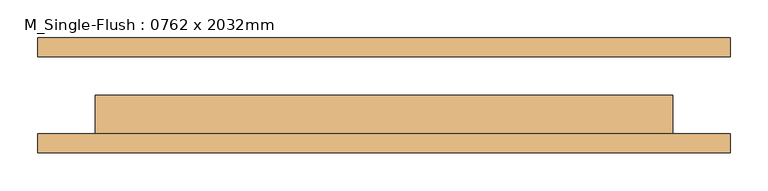
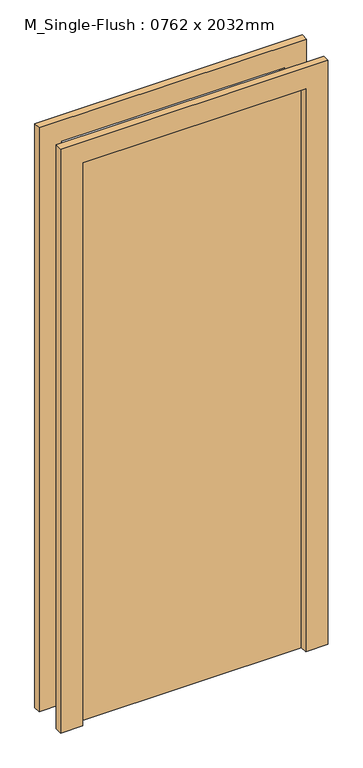
"""IFC4 building model written with IfcOpenShell, lengths in millimetres: door geometry, M_Single-Flush : 0762 x 2032mm."""

from ifc_helpers import new_model, si_unit, frame, origin, origin_with_axes, place, context, project, spatial, polyline, outline, extrude, source, transform, mapped, element, save


def m_single_flush_0762_x_2032mm_63ada305(model_context):
    return source(origin(), model_context, "Body", "SweptSolid", [
        extrude(outline(polyline([(2108.0, -457.0), (0.0, -457.0), (0.0, -381.0), (2032.0, -381.0), (2032.0, 381.0), (0.0, 381.0), (0.0, 457.0), (2108.0, 457.0), (2108.0, -457.0)])), frame((0.0, -75.8, 0.0), z_axis=(0.0, 1.0, 0.0), x_axis=(0.0, 0.0, 1.0)), (0.0, 0.0, 1.0), 25.0),
        extrude(outline(polyline([(2108.0, 457.0), (2108.0, -457.0), (0.0, -457.0), (0.0, -381.0), (2032.0, -381.0), (2032.0, 381.0), (0.0, 381.0), (0.0, 457.0), (2108.0, 457.0)])), frame((0.0, 50.8, 0.0), z_axis=(0.0, 1.0, 0.0), x_axis=(0.0, 0.0, 1.0)), (0.0, 0.0, 1.0), 25.0),
        extrude(outline(polyline([(381.0, 0.2), (381.0, -50.8), (-381.0, -50.8), (-381.0, 0.2), (381.0, 0.2)])), origin_with_axes(), (0.0, 0.0, 1.0), 2032.0),
    ])


if __name__ == "__main__":
    model = new_model("IFC4")
    model_context = context("Model", 3, world=origin())
    ifc_project = project(units=[si_unit("LENGTHUNIT", "METRE", prefix="MILLI")], contexts=[model_context])
    site = spatial("IfcSite", under=ifc_project)
    building = spatial("IfcBuilding", under=site)
    placement = place(None, origin())
    m_single_flush_0762_x_2032mm_shape = m_single_flush_0762_x_2032mm_63ada305(model_context)
    element("IfcDoor", 1, ObjectType="M_Single-Flush : 0762 x 2032mm", at=placement, inside=building, context=model_context, shape_type="MappedRepresentation", body=[
        mapped(m_single_flush_0762_x_2032mm_shape, transform((0.0, 0.0, 0.0), x_axis=(1.0, 0.0, 0.0), y_axis=(0.0, 1.0, 0.0), z_axis=(0.0, 0.0, 1.0))),
    ])
    save(model, "model.ifc")

# Revit data of these elements
# Type "M_Single-Flush : 0762 x 2032mm"
#   Type Mark = "28"
#   Construction Type Id = "MDOOR"
#   Analytic Construction = "Metal"
#   Thickness = 0.167323 ft
#   Thermal Resistance (R) = 0.270117 (m²·K)/W
#   Heat Transfer Coefficient (U) = 3.7021 W/(m²·K)
#   Height = 6.666667 ft
#   Trim Projection Ext = 0.082021 ft
#   Trim Projection Int = 0.082021 ft
#   Trim Width = 0.249344 ft
#   Width = 2.5 ft
#   Define Thermal Properties by = 1
#   Define Thermal Properties by = 1
#   Door Material = Door - Panel
#   Frame Material = Door - Frame
#   Visual Light Transmittance = 0
#   Solar Heat Gain Coefficient = 0
#   Function = (empty or 0)
#   Wall Closure = (empty or 0)
# Element 1 (IfcDoor, "M_Single-Flush : 0762 x 2032mm")
#   Materials on its faces: "Door - Frame", "Door - Panel"
# Materials
#   "Door - Panel": class "Wood", colour RGB 210 159 95, transparency 0, Cost = 0
#   "Door - Frame": colour RGB 118 70 51, transparency 0, Cost = 0
